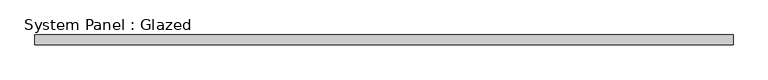
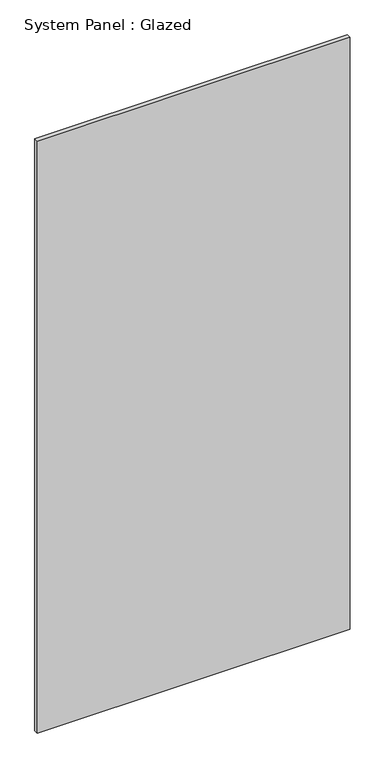
"""IFC4 building model written with IfcOpenShell, lengths in millimetres: plate geometry, System Panel : Glazed."""

from ifc_helpers import new_model, si_unit, origin, origin_with_axes, place, context, project, spatial, polyline, outline, extrude, source, transform, mapped, element, save


def system_panel_glazed_b21aad5f(model_context):
    return source(origin(), model_context, "Body", "SweptSolid", [
        extrude(outline(polyline([(914.4, 19.05), (-914.4, 19.05), (-914.4, 44.45), (914.4, 44.45), (914.4, 19.05)])), origin_with_axes(), (0.0, 0.0, 1.0), 3657.6),
    ])


if __name__ == "__main__":
    model = new_model("IFC4")
    model_context = context("Model", 3, world=origin())
    ifc_project = project(units=[si_unit("LENGTHUNIT", "METRE", prefix="MILLI")], contexts=[model_context])
    site = spatial("IfcSite", under=ifc_project)
    building = spatial("IfcBuilding", under=site)
    placement = place(None, origin())
    system_panel_glazed_shape = system_panel_glazed_b21aad5f(model_context)
    element("IfcPlate", 1, ObjectType="System Panel : Glazed", at=placement, inside=building, context=model_context, shape_type="MappedRepresentation", body=[
        mapped(system_panel_glazed_shape, transform((0.0, 0.0, 0.0), x_axis=(1.0, 0.0, 0.0), y_axis=(0.0, 1.0, 0.0), z_axis=(0.0, 0.0, 1.0))),
    ])
    save(model, "model.ifc")

# Revit data of these elements
# Type "System Panel : Glazed"
#   Construction Type Id = "GSP4R"
#   Analytic Construction = "1/8 in Pilkington single glazing"
#   Visual Light Transmittance = 0.9
#   Solar Heat Gain Coefficient = 0.86
#   Heat Transfer Coefficient (U) = 1.18115 BTU/(h·ft²·°F)
# Element 1 (IfcPlate, "System Panel : Glazed")
#   Materials on its faces: "Glass"
# Materials
#   "Glass": class "Glass", colour RGB 0 128 192, transparency 0.75, Description = "Soda Lime Glass", Cost = 0
